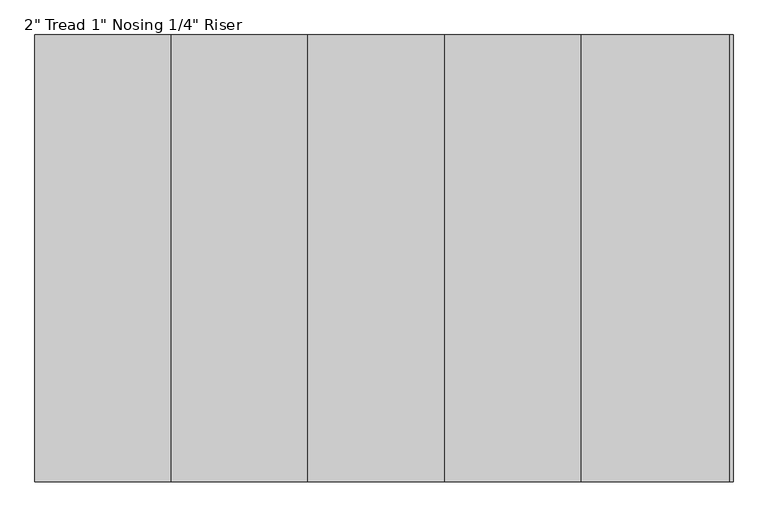
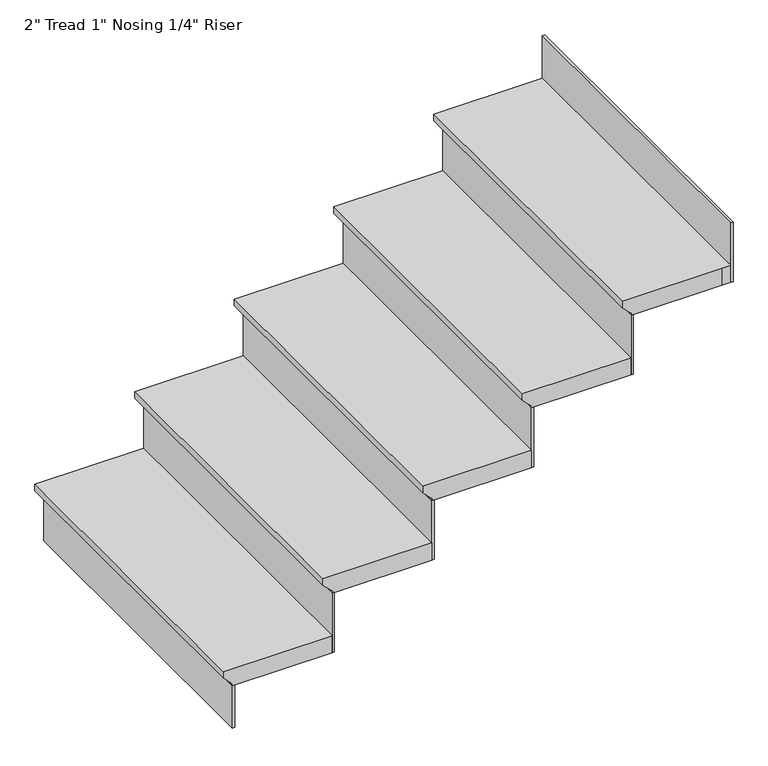
"""IFC4 building model written with IfcOpenShell, lengths in millimetres: stair flight geometry."""

from ifc_helpers import new_model, si_unit, origin, place, context, project, spatial, faceted_brep, source, transform, mapped, element, save


def stair_flight_1ea1789e(model_context):
    return source(origin(), model_context, "Body", "Brep", [
        faceted_brep([(7509.0423568, -10720.6073314, 3510.2131579), (7509.0423568, -10720.6073314, 3529.2631579), (7509.0423568, -9806.2073314, 3529.2631579), (7509.0423568, -9806.2073314, 3510.2131579), (7534.4423568, -10720.6073314, 3484.8131579), (7534.4423568, -9806.2073314, 3484.8131579), (7813.8423568, -10720.6073314, 3529.2631579), (7813.8423568, -9806.2073314, 3529.2631579), (7534.4423568, -9806.2073314, 3478.4631579), (7813.8423568, -9806.2073314, 3478.4631579), (7813.8423568, -10720.6073314, 3478.4631579), (7534.4423568, -10720.6073314, 3478.4631579)], [[[0, 1, 2, 3]], [[4, 0, 3, 5]], [[2, 1, 6, 7]], [[8, 9, 10, 11]], [[2, 7, 9, 8, 5, 3]], [[8, 11, 4, 5]], [[6, 1, 0, 4, 11, 10]], [[7, 6, 10, 9]]]),
        faceted_brep([(7534.4423568, -10720.6073314, 3478.4631579), (7534.4423568, -10720.6073314, 3352.8), (7540.7923568, -10720.6073314, 3352.8), (7540.7923568, -10720.6073314, 3478.4631579), (7534.4423568, -9806.2073314, 3478.4631579), (7540.7923568, -9806.2073314, 3478.4631579), (7540.7923568, -9806.2073314, 3352.8), (7534.4423568, -9806.2073314, 3352.8)], [[[0, 1, 2, 3]], [[4, 5, 6, 7]], [[1, 0, 4, 7]], [[2, 1, 7, 6]], [[3, 2, 6, 5]], [[0, 3, 5, 4]]]),
        faceted_brep([(7813.8423568, -10720.6073314, 3654.9263158), (7813.8423568, -10720.6073314, 3478.4631579), (7820.1923568, -10720.6073314, 3478.4631579), (7820.1923568, -10720.6073314, 3654.9263158), (7813.8423568, -9806.2073314, 3654.9263158), (7820.1923568, -9806.2073314, 3654.9263158), (7820.1923568, -9806.2073314, 3478.4631579), (7813.8423568, -9806.2073314, 3478.4631579)], [[[0, 1, 2, 3]], [[4, 5, 6, 7]], [[1, 0, 4, 7]], [[2, 1, 7, 6]], [[3, 2, 6, 5]], [[0, 3, 5, 4]]]),
        faceted_brep([(7788.4423568, -9806.2073314, 3705.7263158), (7788.4423568, -10720.6073314, 3705.7263158), (8093.2423568, -10720.6073314, 3705.7263158), (8093.2423568, -9806.2073314, 3705.7263158), (7813.8423568, -9806.2073314, 3654.9263158), (8093.2423568, -9806.2073314, 3654.9263158), (8093.2423568, -10720.6073314, 3654.9263158), (7813.8423568, -10720.6073314, 3654.9263158), (7813.8423568, -9806.2073314, 3661.2763158), (7788.4423568, -9806.2073314, 3686.6763158), (7813.8423568, -10720.6073314, 3661.2763158), (7788.4423568, -10720.6073314, 3686.6763158)], [[[0, 1, 2, 3]], [[4, 5, 6, 7]], [[0, 3, 5, 4, 8, 9]], [[4, 7, 10, 8]], [[2, 1, 11, 10, 7, 6]], [[3, 2, 6, 5]], [[11, 1, 0, 9]], [[10, 11, 9, 8]]]),
        faceted_brep([(8093.2423568, -10720.6073314, 3831.3894737), (8093.2423568, -10720.6073314, 3654.9263158), (8099.5923568, -10720.6073314, 3654.9263158), (8099.5923568, -10720.6073314, 3831.3894737), (8093.2423568, -9806.2073314, 3831.3894737), (8099.5923568, -9806.2073314, 3831.3894737), (8099.5923568, -9806.2073314, 3654.9263158), (8093.2423568, -9806.2073314, 3654.9263158)], [[[0, 1, 2, 3]], [[4, 5, 6, 7]], [[1, 0, 4, 7]], [[2, 1, 7, 6]], [[3, 2, 6, 5]], [[0, 3, 5, 4]]]),
        faceted_brep([(8067.8423568, -9806.2073314, 3882.1894737), (8067.8423568, -10720.6073314, 3882.1894737), (8372.6423568, -10720.6073314, 3882.1894737), (8372.6423568, -9806.2073314, 3882.1894737), (8093.2423568, -9806.2073314, 3831.3894737), (8372.6423568, -9806.2073314, 3831.3894737), (8372.6423568, -10720.6073314, 3831.3894737), (8093.2423568, -10720.6073314, 3831.3894737), (8093.2423568, -9806.2073314, 3837.7394737), (8067.8423568, -9806.2073314, 3863.1394737), (8093.2423568, -10720.6073314, 3837.7394737), (8067.8423568, -10720.6073314, 3863.1394737)], [[[0, 1, 2, 3]], [[4, 5, 6, 7]], [[0, 3, 5, 4, 8, 9]], [[4, 7, 10, 8]], [[2, 1, 11, 10, 7, 6]], [[3, 2, 6, 5]], [[11, 1, 0, 9]], [[10, 11, 9, 8]]]),
        faceted_brep([(8372.6423568, -10720.6073314, 4007.8526316), (8372.6423568, -10720.6073314, 3831.3894737), (8378.9923568, -10720.6073314, 3831.3894737), (8378.9923568, -10720.6073314, 4007.8526316), (8372.6423568, -9806.2073314, 4007.8526316), (8378.9923568, -9806.2073314, 4007.8526316), (8378.9923568, -9806.2073314, 3831.3894737), (8372.6423568, -9806.2073314, 3831.3894737)], [[[0, 1, 2, 3]], [[4, 5, 6, 7]], [[1, 0, 4, 7]], [[2, 1, 7, 6]], [[3, 2, 6, 5]], [[0, 3, 5, 4]]]),
        faceted_brep([(8347.2423568, -9806.2073314, 4058.6526316), (8347.2423568, -10720.6073314, 4058.6526316), (8652.0423568, -10720.6073314, 4058.6526316), (8652.0423568, -9806.2073314, 4058.6526316), (8372.6423568, -9806.2073314, 4007.8526316), (8652.0423568, -9806.2073314, 4007.8526316), (8652.0423568, -10720.6073314, 4007.8526316), (8372.6423568, -10720.6073314, 4007.8526316), (8372.6423568, -9806.2073314, 4014.2026316), (8347.2423568, -9806.2073314, 4039.6026316), (8372.6423568, -10720.6073314, 4014.2026316), (8347.2423568, -10720.6073314, 4039.6026316)], [[[0, 1, 2, 3]], [[4, 5, 6, 7]], [[0, 3, 5, 4, 8, 9]], [[4, 7, 10, 8]], [[2, 1, 11, 10, 7, 6]], [[3, 2, 6, 5]], [[11, 1, 0, 9]], [[10, 11, 9, 8]]]),
        faceted_brep([(8931.4423568, -10720.6073314, 4360.7789474), (8931.4423568, -10720.6073314, 4184.3157895), (8937.7923568, -10720.6073314, 4184.3157895), (8937.7923568, -10720.6073314, 4360.7789474), (8931.4423568, -9806.2073314, 4360.7789474), (8937.7923568, -9806.2073314, 4360.7789474), (8937.7923568, -9806.2073314, 4184.3157895), (8931.4423568, -9806.2073314, 4184.3157895)], [[[0, 1, 2, 3]], [[4, 5, 6, 7]], [[1, 0, 4, 7]], [[2, 1, 7, 6]], [[3, 2, 6, 5]], [[0, 3, 5, 4]]]),
        faceted_brep([(8652.0423568, -10720.6073314, 4184.3157895), (8652.0423568, -10720.6073314, 4007.8526316), (8658.3923568, -10720.6073314, 4007.8526316), (8658.3923568, -10720.6073314, 4184.3157895), (8652.0423568, -9806.2073314, 4184.3157895), (8658.3923568, -9806.2073314, 4184.3157895), (8658.3923568, -9806.2073314, 4007.8526316), (8652.0423568, -9806.2073314, 4007.8526316)], [[[0, 1, 2, 3]], [[4, 5, 6, 7]], [[1, 0, 4, 7]], [[2, 1, 7, 6]], [[3, 2, 6, 5]], [[0, 3, 5, 4]]]),
        faceted_brep([(8931.4423568, -9806.2073314, 4235.1157895), (8906.0423568, -9806.2073314, 4235.1157895), (8626.6423568, -9806.2073314, 4235.1157895), (8626.6423568, -10720.6073314, 4235.1157895), (8906.0423568, -10720.6073314, 4235.1157895), (8931.4423568, -10720.6073314, 4235.1157895), (8906.0423568, -9806.2073314, 4184.3157895), (8931.4423568, -9806.2073314, 4184.3157895), (8931.4423568, -10720.6073314, 4184.3157895), (8906.0423568, -10720.6073314, 4184.3157895), (8652.0423568, -10720.6073314, 4184.3157895), (8652.0423568, -9806.2073314, 4184.3157895), (8652.0423568, -9806.2073314, 4190.6657895), (8626.6423568, -9806.2073314, 4216.0657895), (8652.0423568, -10720.6073314, 4190.6657895), (8626.6423568, -10720.6073314, 4216.0657895)], [[[0, 1, 2, 3, 4, 5]], [[6, 7, 8, 9, 10, 11]], [[1, 0, 7, 6]], [[2, 1, 6, 11, 12, 13]], [[11, 10, 14, 12]], [[4, 3, 15, 14, 10, 9]], [[5, 4, 9, 8]], [[0, 5, 8, 7]], [[15, 3, 2, 13]], [[14, 15, 13, 12]]]),
    ])


if __name__ == "__main__":
    model = new_model("IFC4")
    model_context = context("Model", 3, world=origin())
    ifc_project = project(units=[si_unit("LENGTHUNIT", "METRE", prefix="MILLI")], contexts=[model_context])
    site = spatial("IfcSite", under=ifc_project)
    building = spatial("IfcBuilding", under=site)
    placement = place(None, origin())
    stair_flight_shape = stair_flight_1ea1789e(model_context)
    element("IfcStairFlight", 1, ObjectType="2\" Tread 1\" Nosing 1/4\" Riser", at=placement, inside=building, context=model_context, shape_type="MappedRepresentation", body=[
        mapped(stair_flight_shape, transform((0.0, 0.0, 0.0), x_axis=(1.0, 0.0, 0.0), y_axis=(0.0, 1.0, 0.0), z_axis=(0.0, 0.0, 1.0))),
    ])
    save(model, "model.ifc")

# Revit data of these elements
# Element 1 (IfcStairFlight, "2\" Tread 1\" Nosing 1/4\" Riser")
#   Materials on its faces: "MARBLE STAIRS 6\""
# Materials
#   "MARBLE STAIRS 6\"": class "Generic", colour RGB 120 120 120, transparency 0, Cost = 0
